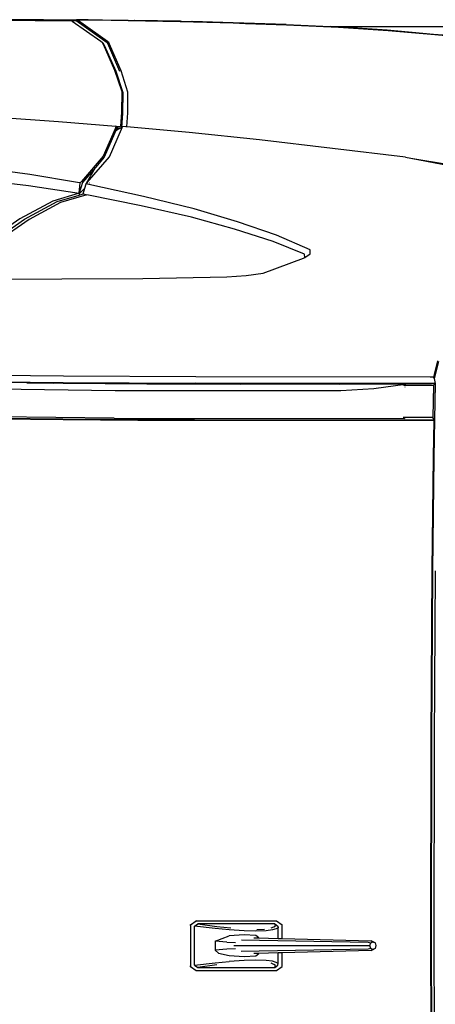
# Model space of a CAD drawing. Units: inches. Extents: x 22042254 to 25404563, y 17568978 to 17626777.
# Tile 8 of 45: x 22042256.1597 to 22042256.4081, y 17568978.1821 to 17568978.7711. Entities that reach past the tile are written whole.
import ezdxf

# ---------------------------------------------------------------- set-up
doc = ezdxf.new("R2010")
doc.units = ezdxf.units.IN
doc.header["$MEASUREMENT"] = 0
doc.layers.add('A-SITE-VEHI', color=8, linetype='Continuous', lineweight=18)
doc.layers.add('Edges', color=250, linetype='Continuous')

# ---------------------------------------------------------------- blocks, each defined once
blk = doc.blocks.new('Nissan Qashqai pl')
at = {"layer": 'Edges'}
for p, q in [((11.05474, 11.92208), (11.05507, 12.12031)), ((11.05537, 11.92208), (11.05571, 12.1202)), ((11.0586, 12.11975), (11.05827, 11.92208)), ((10.8228, 11.94208), (10.82239, 11.94208)), ((10.8228, 11.94208), (10.82834, 11.94608)), ((10.8228, 11.90208), (10.8228, 11.94208)), ((10.82696, 11.94083), (10.83007, 11.94308)), ((10.82696, 11.94083), (10.82696, 11.90333)), ((10.82696, 11.94083), (10.84666, 11.93861)), ((10.82794, 11.94608), (10.82834, 11.94608)), ((10.82834, 11.94608), (10.90603, 11.94608)), ((10.84833, 11.9406), (10.83007, 11.94308)), ((10.83007, 11.94308), (10.9043, 11.94308)), ((10.90348, 11.94026), (10.90076, 11.93914)), ((10.90503, 11.94137), (10.90348, 11.94026)), ((10.9043, 11.94308), (10.90741, 11.94083)), ((10.9043, 11.94308), (10.90503, 11.94137)), ((10.90744, 11.9393), (10.90565, 11.93837)), ((10.90603, 11.94608), (10.91157, 11.94208)), ((10.90741, 11.94083), (10.90744, 11.9393)), ((10.90744, 11.9393), (10.90744, 11.92915)), ((10.91157, 11.94208), (10.91157, 11.92904)), ((10.84666, 11.93861), (10.86027, 11.93735)), ((10.85007, 11.92947), (10.86027, 11.93157)), ((10.8746, 11.93634), (10.86027, 11.93735)), ((10.86027, 11.93157), (10.8746, 11.93265)), ((10.88611, 11.93611), (10.8746, 11.93634)), ((10.8746, 11.93265), (10.88611, 11.93193)), ((10.889, 11.92962), (10.88395, 11.92975)), ((10.89593, 11.93645), (10.88611, 11.93611)), ((10.88611, 11.93193), (10.889, 11.92962)), ((10.90744, 11.92915), (10.889, 11.92962)), ((10.90215, 11.93722), (10.89593, 11.93645)), ((10.90565, 11.93837), (10.90215, 11.93722)), ((10.84666, 11.92634), (10.85007, 11.92947)), ((10.84666, 11.91782), (10.84666, 11.92634)), ((10.85787, 11.92547), (10.84666, 11.92634)), ((10.86624, 11.92503), (10.85787, 11.92547)), ((10.86474, 11.92208), (10.99603, 11.92208)), ((10.99456, 11.92544), (10.87195, 11.92764)), ((10.91157, 11.92904), (10.90744, 11.92915)), ((10.99731, 11.92683), (10.91157, 11.92904)), ((10.99691, 11.92468), (10.99456, 11.92544)), ((10.99691, 11.92468), (10.99603, 11.92208)), ((10.99603, 11.92208), (10.99691, 11.91949)), ((10.99903, 11.92575), (10.99691, 11.92468)), ((10.99731, 11.92683), (11.00007, 11.92544)), ((10.99903, 11.92575), (10.99731, 11.92683)), ((11.00116, 11.92468), (10.99903, 11.92575)), ((11.00116, 11.92468), (11.00007, 11.92544)), ((11.00204, 11.92208), (11.00116, 11.92468)), ((11.00116, 11.91949), (11.00204, 11.92208)), ((11.05507, 11.72385), (11.05474, 11.92208)), ((11.05571, 11.72396), (11.05537, 11.92208)), ((11.05827, 11.92208), (11.0586, 11.72441)), ((10.85787, 11.91869), (10.84666, 11.91782)), ((10.84666, 11.91782), (10.86027, 11.91259)), ((10.85787, 11.91869), (10.86624, 11.91913)), ((10.8746, 11.91151), (10.86027, 11.91259)), ((10.87225, 11.91653), (10.99456, 11.91872)), ((10.88611, 11.91223), (10.8746, 11.91151)), ((10.88395, 11.91441), (10.889, 11.91454)), ((10.889, 11.91454), (10.88611, 11.91223)), ((10.889, 11.91454), (10.90744, 11.91502)), ((10.90744, 11.91502), (10.91157, 11.91512)), ((10.90744, 11.91502), (10.90744, 11.90486)), ((10.91157, 11.91512), (10.99731, 11.91733)), ((10.91157, 11.91512), (10.91157, 11.90208)), ((10.99456, 11.91872), (10.99691, 11.91949)), ((10.99691, 11.91949), (10.99903, 11.91841)), ((11.00007, 11.91872), (10.99731, 11.91733)), ((10.99731, 11.91733), (10.99903, 11.91841)), ((10.99903, 11.91841), (10.99963, 11.91871)), ((10.99963, 11.91871), (11.00116, 11.91949)), ((11.00007, 11.91872), (10.99963, 11.91871)), ((11.00116, 11.91949), (11.00007, 11.91872)), ((10.82239, 11.90208), (10.8228, 11.90208)), ((10.8228, 11.90208), (10.82834, 11.89808)), ((10.84666, 11.90555), (10.82696, 11.90333)), ((10.82696, 11.90333), (10.83007, 11.90108)), ((10.83007, 11.90108), (10.84833, 11.90356)), ((10.9043, 11.90108), (10.83007, 11.90108)), ((10.86027, 11.90681), (10.84666, 11.90555)), ((10.84833, 11.90356), (10.86193, 11.905)), ((10.8746, 11.90782), (10.86027, 11.90681)), ((10.88611, 11.90805), (10.8746, 11.90782)), ((10.89593, 11.90771), (10.88611, 11.90805)), ((10.88709, 11.90634), (10.89442, 11.90601)), ((10.90215, 11.90694), (10.89593, 11.90771)), ((10.90076, 11.90502), (10.90348, 11.9039)), ((10.90565, 11.90579), (10.90215, 11.90694)), ((10.90348, 11.9039), (10.90503, 11.90279)), ((10.9043, 11.90108), (10.90741, 11.90333)), ((10.90503, 11.90279), (10.9043, 11.90108)), ((10.90744, 11.90486), (10.90565, 11.90579)), ((10.90603, 11.89808), (10.91157, 11.90208)), ((10.90741, 11.90333), (10.90744, 11.90486)), ((10.90741, 11.90333), (10.90741, 11.90484)), ((10.82834, 11.89808), (10.82794, 11.89808)), ((10.82834, 11.89808), (10.90603, 11.89808)), ((11.05596, 11.55904), (11.05507, 11.72385)), ((11.0566, 11.5593), (11.05571, 11.72396)), ((11.0586, 11.72441), (11.05947, 11.55994)), ((11.05722, 11.44991), (11.05596, 11.55904)), ((11.05785, 11.45038), (11.0566, 11.5593)), ((11.05789, 11.4146), (11.05722, 11.44991)), ((11.05854, 11.41419), (11.05785, 11.45038)), ((10.69961, 11.41337), (10.55607, 11.41187)), ((10.5563, 11.41232), (10.69989, 11.41381)), ((10.7493, 11.41253), (10.62233, 11.41086)), ((10.77221, 11.41378), (10.69961, 11.41337)), ((10.69989, 11.41381), (10.77221, 11.4142)), ((10.7493, 11.41253), (11.02943, 11.41262)), ((10.77221, 11.4142), (10.78885, 11.41429)), ((10.77221, 11.4142), (10.77221, 11.41378)), ((10.78885, 11.41387), (10.77221, 11.41378)), ((10.78885, 11.41429), (10.79225, 11.41431)), ((10.78885, 11.41387), (10.78885, 11.41429)), ((10.79225, 11.41389), (10.78885, 11.41387)), ((10.79225, 11.41431), (10.79328, 11.41432)), ((10.79225, 11.41389), (10.79225, 11.41431)), ((10.79328, 11.4139), (10.79225, 11.41389)), ((10.79328, 11.41432), (10.82704, 11.4145)), ((10.79328, 11.4139), (10.79328, 11.41432)), ((10.82673, 11.41408), (10.79328, 11.4139)), ((10.82673, 11.41408), (11.05854, 11.41419)), ((10.82704, 11.4145), (11.05789, 11.4146)), ((11.02945, 11.41183), (11.02814, 11.41183)), ((11.02944, 11.41252), (11.02943, 11.41262)), ((11.05683, 11.41184), (11.02945, 11.41183)), ((11.02945, 11.41162), (11.02945, 11.41183)), ((11.05854, 11.41419), (11.05683, 11.41184)), ((11.05743, 11.38044), (11.05683, 11.41184)), ((11.05854, 11.41419), (11.05789, 11.4146)), ((11.05921, 11.37886), (11.05854, 11.41419)), ((10.55662, 11.37645), (10.69998, 11.37799)), ((10.6649, 11.37825), (10.55757, 11.37665)), ((10.6649, 11.37825), (10.58658, 11.37719)), ((10.62366, 11.38388), (10.75022, 11.38554)), ((10.69078, 11.37855), (10.6649, 11.37825)), ((10.6649, 11.37825), (10.67717, 11.37844)), ((10.69658, 11.37873), (10.67717, 11.37844)), ((10.67717, 11.37844), (10.69078, 11.37855)), ((10.69913, 11.37864), (10.69078, 11.37855)), ((10.71439, 11.37882), (10.69658, 11.37873)), ((10.69986, 11.37862), (10.69913, 11.37864)), ((10.69986, 11.37862), (10.78083, 11.37927)), ((10.71439, 11.37882), (10.69986, 11.37862)), ((10.69998, 11.37799), (10.82786, 11.37874)), ((10.72388, 11.37887), (10.71439, 11.37882)), ((10.72479, 11.37891), (10.72388, 11.37887)), ((10.78083, 11.37927), (10.72479, 11.37891)), ((10.75022, 11.38554), (10.96805, 11.38566)), ((10.78083, 11.37927), (10.8711, 11.37956)), ((10.94306, 11.3796), (10.82786, 11.37874)), ((10.82786, 11.37874), (11.05524, 11.37886)), ((10.96142, 11.37881), (10.82786, 11.37874)), ((10.89604, 11.37957), (10.8711, 11.37956)), ((10.90974, 11.3796), (10.89604, 11.37957)), ((10.94306, 11.3796), (10.90974, 11.3796)), ((10.94785, 11.37963), (10.94306, 11.3796)), ((10.9491, 11.37964), (10.94785, 11.37963)), ((10.96679, 11.37961), (10.9491, 11.37964)), ((10.96142, 11.37881), (10.96679, 11.37961)), ((10.97113, 11.37881), (10.96142, 11.37881)), ((10.96679, 11.37961), (10.96696, 11.37964)), ((10.97653, 11.37962), (10.96696, 11.37964)), ((10.96805, 11.38566), (10.99996, 11.38365)), ((10.97653, 11.37962), (10.97113, 11.37881)), ((10.97664, 11.37882), (10.97113, 11.37881)), ((10.98248, 11.37964), (10.97653, 11.37962)), ((10.97653, 11.37962), (10.97664, 11.37882)), ((11.05921, 11.37886), (10.97664, 11.37882)), ((11.03007, 11.37965), (10.98248, 11.37964)), ((10.99996, 11.38365), (11.03007, 11.37965)), ((11.02869, 11.38043), (11.03005, 11.38043)), ((11.03005, 11.38025), (11.02923, 11.38024)), ((11.03002, 11.38217), (11.03001, 11.38239)), ((11.03005, 11.38043), (11.05544, 11.38044)), ((11.05544, 11.38044), (11.03005, 11.38025)), ((11.03005, 11.38025), (11.03005, 11.38043)), ((11.03007, 11.37965), (11.03005, 11.38025)), ((11.05544, 11.38044), (11.05743, 11.38044)), ((11.05921, 11.37886), (11.05743, 11.38044)), ((11.05822, 11.37418), (11.05921, 11.37886)), ((10.7004, 11.37196), (10.55723, 11.37045)), ((10.82794, 11.37265), (10.7004, 11.37196)), ((11.05437, 11.37279), (10.82794, 11.37265)), ((11.05754, 11.37277), (11.05437, 11.37279)), ((11.05822, 11.37418), (11.05754, 11.37277)), ((11.05807, 11.37037), (11.05754, 11.37277)), ((11.06139, 11.35691), (11.05807, 11.37037)), ((11.06236, 11.3576), (11.05822, 11.37418)), ((10.58925, 11.27827), (10.69879, 11.27793)), ((10.69879, 11.27793), (10.77686, 11.27742)), ((10.77686, 11.27742), (10.85804, 11.27587)), ((10.85804, 11.27587), (10.87661, 11.27449)), ((10.87661, 11.27449), (10.89318, 11.27219)), ((10.89318, 11.27219), (10.932, 11.25799)), ((10.932, 11.25799), (10.93345, 11.25704)), ((10.93345, 11.25704), (10.93299, 11.25409)), ((10.93345, 11.25704), (10.93862, 11.25365)), ((10.65826, 11.2197), (10.62146, 11.24557)), ((10.62607, 11.24576), (10.6627, 11.22001)), ((10.6671, 11.22032), (10.63062, 11.24593)), ((10.93299, 11.25409), (10.90264, 11.24169)), ((10.9384, 11.24966), (10.90591, 11.23547)), ((10.93862, 11.25365), (10.9384, 11.24966)), ((10.90264, 11.24169), (10.86528, 11.22973)), ((10.90591, 11.23547), (10.86821, 11.22258)), ((10.86528, 11.22973), (10.82385, 11.21811)), ((10.69003, 11.20277), (10.65826, 11.2197)), ((10.6627, 11.22001), (10.6943, 11.20317)), ((10.69755, 11.20409), (10.6671, 11.22032)), ((10.82385, 11.21811), (10.77536, 11.20713)), ((10.86821, 11.22258), (10.82645, 11.21003)), ((10.77536, 11.20713), (10.72279, 11.1965)), ((10.82645, 11.21003), (10.77763, 11.19817)), ((10.71545, 11.19515), (10.69003, 11.20277)), ((10.6943, 11.20317), (10.71545, 11.19687)), ((10.72279, 11.1965), (10.69755, 11.20409)), ((10.77763, 11.19817), (10.72473, 11.18666)), ((10.61435, 11.18131), (10.66642, 11.18754)), ((10.66642, 11.18754), (10.71545, 11.19515)), ((10.71545, 11.1957), (10.71545, 11.19687)), ((10.71545, 11.19687), (10.71925, 11.19574)), ((10.72089, 11.19018), (10.71545, 11.1957)), ((10.71545, 11.19515), (10.71545, 11.1957)), ((10.71859, 11.18483), (10.71545, 11.19515)), ((10.71545, 11.19515), (10.71653, 11.1851)), ((10.71925, 11.19574), (10.72279, 11.1965)), ((10.71925, 11.19574), (10.72089, 11.19018)), ((10.72089, 11.19018), (10.7221, 11.18607)), ((10.71369, 11.18463), (10.6678, 11.17696)), ((10.71653, 11.1851), (10.71369, 11.18463)), ((10.71766, 11.18379), (10.71653, 11.1851)), ((10.73867, 11.15929), (10.71766, 11.18379)), ((10.73119, 11.17009), (10.71859, 11.18483)), ((10.7221, 11.18607), (10.72224, 11.1859)), ((10.7222, 11.18605), (10.7221, 11.18607)), ((10.72473, 11.18666), (10.7222, 11.18605)), ((10.7222, 11.18605), (10.72224, 11.1859)), ((10.72224, 11.1859), (10.72325, 11.18477)), ((10.72224, 11.1859), (10.72238, 11.18545)), ((10.72238, 11.18545), (10.73119, 11.17009)), ((10.72325, 11.18477), (10.72282, 11.18593)), ((10.72325, 11.18477), (10.74486, 11.15985)), ((10.72567, 11.18531), (10.72556, 11.18542)), ((11.03575, 11.16129), (11.1598, 11.18473)), ((10.6678, 11.17696), (10.61519, 11.17018)), ((10.73966, 11.16018), (10.73119, 11.17009)), ((11.04919, 11.16347), (11.13359, 11.17719)), ((10.75013, 11.13275), (10.73867, 11.15929)), ((10.75073, 11.1344), (10.73966, 11.16018)), ((10.74486, 11.15985), (10.75628, 11.13325)), ((11.03041, 11.16033), (10.88962, 11.14337)), ((11.03041, 11.16033), (11.03575, 11.16129)), ((11.03575, 11.16129), (11.04905, 11.16345)), ((11.04919, 11.16347), (11.04905, 11.16345)), ((10.88962, 11.14337), (10.82176, 11.13649)), ((10.75069, 11.13095), (10.75013, 11.13275)), ((10.75097, 11.13097), (10.75069, 11.13095)), ((10.75092, 11.13018), (10.75069, 11.13095)), ((10.75111, 11.13351), (10.75073, 11.1344)), ((10.75073, 11.1344), (10.75244, 11.13354)), ((10.75224, 11.13107), (10.75092, 11.13018)), ((10.75161, 11.13102), (10.75092, 11.13018)), ((10.75189, 11.13136), (10.75111, 11.13351)), ((10.75189, 11.13136), (10.75161, 11.13102)), ((10.75224, 11.13107), (10.75161, 11.13102)), ((10.75256, 11.13175), (10.75189, 11.13136)), ((10.75535, 11.13074), (10.75224, 11.13107)), ((10.75244, 11.13354), (10.75256, 11.13175)), ((10.75244, 11.13354), (10.75565, 11.13194)), ((10.75322, 11.13213), (10.75256, 11.13175)), ((10.75256, 11.13175), (10.75259, 11.13145)), ((10.75565, 11.13194), (10.75322, 11.13213)), ((10.75627, 11.1169), (10.75535, 11.13074)), ((10.75565, 11.13194), (10.75612, 11.1317)), ((10.75631, 11.13154), (10.75612, 11.1317)), ((10.75612, 11.1317), (10.75629, 11.13169)), ((10.75628, 11.13189), (10.75614, 11.1319)), ((10.75628, 11.13325), (10.75689, 11.13167)), ((10.75629, 11.13169), (10.75628, 11.13189)), ((10.75629, 11.13169), (10.75689, 11.13167)), ((10.7569, 11.13164), (10.75629, 11.13169)), ((10.75631, 11.13154), (10.75629, 11.13169)), ((10.75723, 11.11783), (10.75631, 11.13154)), ((10.75727, 11.1307), (10.75631, 11.13154)), ((10.75689, 11.13167), (10.7569, 11.13164)), ((10.7569, 11.13164), (10.75727, 11.1307)), ((10.76042, 11.13099), (10.75727, 11.1307)), ((10.76145, 11.13107), (10.76042, 11.13099)), ((10.82176, 11.13649), (10.76145, 11.13107)), ((10.76145, 11.13107), (10.76229, 11.1173)), ((10.63183, 11.12133), (10.69546, 11.12574)), ((10.69546, 11.12574), (10.75092, 11.13018)), ((10.75648, 11.09691), (10.75627, 11.1169)), ((10.75747, 11.09792), (10.75723, 11.11783)), ((10.76229, 11.1173), (10.76258, 11.09741)), ((10.74965, 11.07628), (10.75648, 11.09691)), ((10.7507, 11.07729), (10.75747, 11.09792)), ((10.76258, 11.09741), (10.75592, 11.07672)), ((10.73846, 11.051), (10.74965, 11.07628)), ((10.73956, 11.05193), (10.7507, 11.07729)), ((10.75486, 11.07758), (10.74298, 11.05028)), ((10.75592, 11.07672), (10.74477, 11.05114)), ((10.70875, 11.02887), (10.7363, 11.0483)), ((10.74241, 11.04987), (10.71254, 11.02855)), ((10.74291, 11.04852), (10.7148, 11.02842)), ((10.7363, 11.0483), (10.73758, 11.04917)), ((10.73869, 11.05016), (10.73758, 11.04917)), ((10.73758, 11.04917), (10.73776, 11.04954)), ((10.73776, 11.04954), (10.73846, 11.051)), ((10.73776, 11.04954), (10.73792, 11.04965)), ((10.73869, 11.05016), (10.73956, 11.05193)), ((10.74241, 11.04987), (10.74298, 11.05028)), ((10.74324, 11.04877), (10.74291, 11.04852)), ((10.74292, 11.04876), (10.74324, 11.04877)), ((10.74404, 11.04936), (10.74324, 11.04877)), ((10.74477, 11.05114), (10.74404, 11.04936)), ((11.01272, 11.03746), (10.9649, 11.03441)), ((10.9657, 11.03466), (11.01381, 11.03772)), ((11.05762, 11.04159), (11.01272, 11.03746)), ((11.01381, 11.03772), (11.05899, 11.04188)), ((11.07977, 11.04339), (11.05762, 11.04159)), ((11.05899, 11.04188), (11.07681, 11.04337)), ((10.61514, 11.02827), (10.66445, 11.02801)), ((10.66511, 11.02743), (10.61756, 11.02773)), ((10.66445, 11.02801), (10.7078, 11.02821)), ((10.67702, 11.02746), (10.66511, 11.02743)), ((10.70817, 11.02853), (10.67289, 11.02845)), ((10.68004, 11.02743), (10.67702, 11.02746)), ((10.68094, 11.02743), (10.68004, 11.02743)), ((10.68094, 11.02743), (10.71276, 11.02755)), ((10.7078, 11.02821), (10.70826, 11.02853)), ((10.70817, 11.02853), (10.7078, 11.02821)), ((10.70855, 11.02887), (10.70817, 11.02853)), ((10.70826, 11.02853), (10.70817, 11.02853)), ((10.70826, 11.02853), (10.70875, 11.02887)), ((10.71254, 11.02855), (10.70826, 11.02853)), ((10.71464, 11.02857), (10.71254, 11.02855)), ((10.71254, 11.02855), (10.71391, 11.02779)), ((10.71338, 11.02755), (10.71276, 11.02755)), ((10.76246, 11.02806), (10.71338, 11.02755)), ((10.72402, 11.02755), (10.71338, 11.02755)), ((10.7148, 11.02842), (10.71391, 11.02779)), ((10.76281, 11.02832), (10.71391, 11.02779)), ((10.72402, 11.02755), (10.76848, 11.02806)), ((10.76281, 11.02806), (10.76246, 11.02806)), ((10.76281, 11.02832), (10.81307, 11.02924)), ((10.76281, 11.02806), (10.81313, 11.029)), ((10.76883, 11.02806), (10.76848, 11.02806)), ((10.81313, 11.029), (10.76883, 11.02806)), ((10.81307, 11.02924), (10.86443, 11.03061)), ((10.81319, 11.029), (10.81313, 11.029)), ((10.81319, 11.029), (10.81393, 11.02902)), ((10.81418, 11.029), (10.81393, 11.02902)), ((10.81424, 11.029), (10.81418, 11.029)), ((10.81424, 11.029), (10.82415, 11.02929)), ((10.82419, 11.02929), (10.82415, 11.02929)), ((10.82464, 11.02931), (10.82419, 11.02929)), ((10.8642, 11.03037), (10.82464, 11.02931)), ((10.91525, 11.03213), (10.8642, 11.03037)), ((10.86421, 11.03053), (10.8759, 11.031)), ((10.86443, 11.03061), (10.8759, 11.031)), ((10.8759, 11.031), (10.91576, 11.03237)), ((10.91525, 11.03213), (10.95773, 11.03408)), ((10.91576, 11.03237), (10.9657, 11.03466)), ((10.9649, 11.03441), (10.95773, 11.03408)), ((10.95773, 11.03408), (11.12828, 11.03408))]:
    blk.add_line(p, q, dxfattribs=at)
blk = doc.blocks.new('CAR')
blk.add_blockref('Nissan Qashqai pl', (-9.74328, -11.91512))

msp = doc.modelspace()

# ---------------------------------------------------------------- block references
at = {"layer": 'A-SITE-VEHI', "xscale": -0.6191396643141144, "yscale": 0.6191396643141144, "zscale": 0.6191396643141144, "rotation": 180}
msp.add_blockref('CAR', (22042255.59333, 17568978.22147), dxfattribs=at)

doc.saveas('drawing.dxf')
